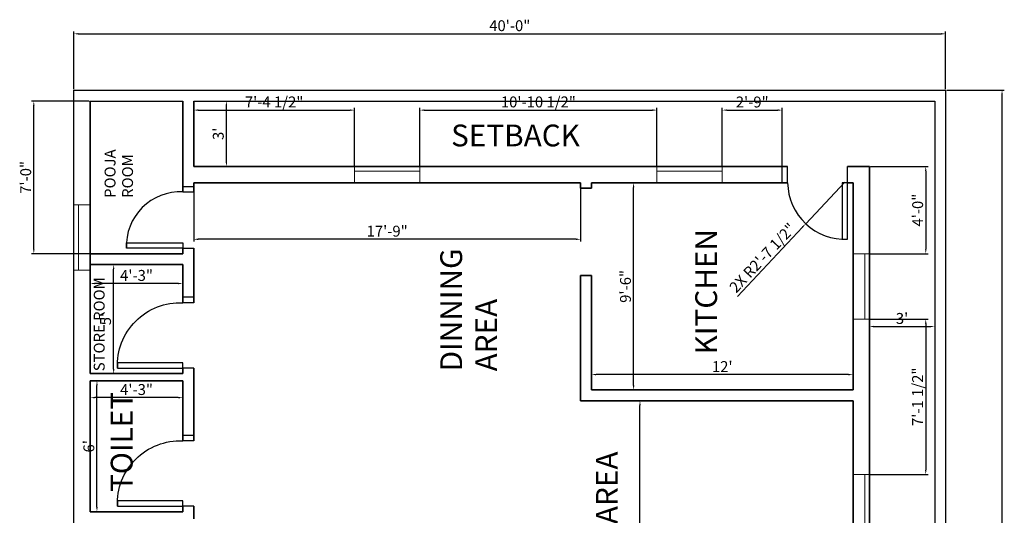
# Model space of a CAD drawing. Units: inches. Extents: x 2641 to 3210, y 2696 to 4064.
# Tile 2 of 4: x 2650 to 3192, y 3095 to 3367. Entities that reach past the tile are written whole.
import ezdxf

# ---------------------------------------------------------------- set-up
doc = ezdxf.new("R2010")
doc.units = ezdxf.units.IN
for name, color, linetype, lineweight in [('A-ANNO-DIMS', 2, 'Continuous', 18), ('A-AREA-IDEN', 7, 'Continuous', 18), ('A-DOOR', 3, 'Continuous', 25), ('A-GLAZ', 4, 'Continuous', 18), ('A-WALL', 7, 'Continuous', 35), ('C-PROP', 8, 'Continuous', 25)]:
    doc.layers.add(name, color=color, linetype=linetype, lineweight=lineweight)
doc.styles.get("Standard").update_dxf_attribs({"font": 'arial.ttf'})
doc.dimstyles.new('ISO-25', dxfattribs={"dimtxt": 6, "dimasz": 2.5, "dimexe": 1.25, "dimexo": 0.625, "dimtad": 1, "dimdec": 1, "dimlunit": 3, "dimtxsty": 'Standard', "dimcen": 2.5, "dimadec": 0, "dimazin": 0, "dimtfac": 1, "dimtdec": 1, "dimtmove": 0, "dimatfit": 3, "dimfxl": 1, "dimarcsym": 0})

# ---------------------------------------------------------------- blocks, each defined once
blk = doc.blocks.new('*D8')
at = {"layer": 'A-ANNO-DIMS', "color": 0, "lineweight": -2, "transparency": 16777216}
for p, q in [((2689.25, 3168.55), (2693.59, 3168.55)), ((2692.34, 3099.05), (2692.34, 3166.05)), ((2689.25, 3096.55), (2693.59, 3096.55))]:
    blk.add_line(p, q, dxfattribs=at)
at = {"layer": 'A-ANNO-DIMS', "color": 0, "transparency": 16777216}
for points in [[(2691.93, 3166.05), (2692.76, 3166.05), (2692.34, 3168.55)], [(2691.93, 3099.05), (2692.76, 3099.05), (2692.34, 3096.55)]]:
    blk.add_solid(points, dxfattribs=at)
at = {"layer": 'Defpoints', "color": 0, "transparency": 16777216}
for p in [(2688.63, 3168.55), (2692.34, 3168.55), (2688.63, 3096.55)]:
    blk.add_point(p, dxfattribs=at)
at = {"layer": 'A-ANNO-DIMS', "color": 0, "transparency": 16777216, "insert": (2688.65, 3132.55), "char_height": 6, "attachment_point": 5, "rotation": 90}
blk.add_mtext("6'", dxfattribs=at)
blk = doc.blocks.new('*D9')
at = {"layer": 'A-ANNO-DIMS', "color": 0, "lineweight": -2, "transparency": 16777216}
for p, q in [((2688.63, 3167.92), (2688.63, 3158.06)), ((2739.63, 3167.92), (2739.63, 3158.06)), ((2737.13, 3159.31), (2691.13, 3159.31))]:
    blk.add_line(p, q, dxfattribs=at)
at = {"layer": 'A-ANNO-DIMS', "color": 0, "transparency": 16777216}
for points in [[(2691.13, 3159.73), (2691.13, 3158.89), (2688.63, 3159.31)], [(2737.13, 3159.73), (2737.13, 3158.89), (2739.63, 3159.31)]]:
    blk.add_solid(points, dxfattribs=at)
at = {"layer": 'Defpoints', "color": 0, "transparency": 16777216}
for p in [(2688.63, 3168.55), (2739.63, 3168.55), (2688.63, 3159.31)]:
    blk.add_point(p, dxfattribs=at)
at = {"layer": 'A-ANNO-DIMS', "color": 0, "transparency": 16777216, "insert": (2714.13, 3163), "char_height": 6, "attachment_point": 5}
blk.add_mtext('4\'-3"', dxfattribs=at)
blk = doc.blocks.new('*D10')
at = {"layer": 'A-ANNO-DIMS', "color": 0, "lineweight": -2, "transparency": 16777216}
for p, q in [((2689.25, 3232.55), (2702.79, 3232.55)), ((2701.54, 3175.05), (2701.54, 3230.05)), ((2689.25, 3172.55), (2702.79, 3172.55))]:
    blk.add_line(p, q, dxfattribs=at)
at = {"layer": 'A-ANNO-DIMS', "color": 0, "transparency": 16777216}
for points in [[(2701.12, 3230.05), (2701.96, 3230.05), (2701.54, 3232.55)], [(2701.12, 3175.05), (2701.96, 3175.05), (2701.54, 3172.55)]]:
    blk.add_solid(points, dxfattribs=at)
at = {"layer": 'Defpoints', "color": 0, "transparency": 16777216}
for p in [(2688.63, 3232.55), (2701.54, 3232.55), (2688.63, 3172.55)]:
    blk.add_point(p, dxfattribs=at)
at = {"layer": 'A-ANNO-DIMS', "color": 0, "transparency": 16777216, "insert": (2697.86, 3202.55), "char_height": 6, "attachment_point": 5, "rotation": 90}
blk.add_mtext("5'", dxfattribs=at)
blk = doc.blocks.new('*D11')
at = {"layer": 'A-ANNO-DIMS', "color": 0, "lineweight": -2, "transparency": 16777216}
for p, q in [((2688.63, 3231.92), (2688.63, 3220.89)), ((2739.63, 3231.92), (2739.63, 3220.89)), ((2737.13, 3222.14), (2691.13, 3222.14))]:
    blk.add_line(p, q, dxfattribs=at)
at = {"layer": 'A-ANNO-DIMS', "color": 0, "transparency": 16777216}
for points in [[(2691.13, 3222.56), (2691.13, 3221.72), (2688.63, 3222.14)], [(2737.13, 3222.56), (2737.13, 3221.72), (2739.63, 3222.14)]]:
    blk.add_solid(points, dxfattribs=at)
at = {"layer": 'Defpoints', "color": 0, "transparency": 16777216}
for p in [(2688.63, 3232.55), (2739.63, 3232.55), (2688.63, 3222.14)]:
    blk.add_point(p, dxfattribs=at)
at = {"layer": 'A-ANNO-DIMS', "color": 0, "transparency": 16777216, "insert": (2714.13, 3225.83), "char_height": 6, "attachment_point": 5}
blk.add_mtext('4\'-3"', dxfattribs=at)
blk = doc.blocks.new('*D12')
at = {"layer": 'A-ANNO-DIMS', "color": 0, "lineweight": -2, "transparency": 16777216}
for p, q in [((2965.25, 3277.55), (2989.06, 3277.55)), ((2987.81, 3166.05), (2987.81, 3275.05)), ((2965.25, 3163.55), (2989.06, 3163.55))]:
    blk.add_line(p, q, dxfattribs=at)
at = {"layer": 'A-ANNO-DIMS', "color": 0, "transparency": 16777216}
for points in [[(2987.4, 3275.05), (2988.23, 3275.05), (2987.81, 3277.55)], [(2987.4, 3166.05), (2988.23, 3166.05), (2987.81, 3163.55)]]:
    blk.add_solid(points, dxfattribs=at)
at = {"layer": 'Defpoints', "color": 0, "transparency": 16777216}
for p in [(2964.63, 3277.55), (2987.81, 3277.55), (2964.63, 3163.55)]:
    blk.add_point(p, dxfattribs=at)
at = {"layer": 'A-ANNO-DIMS', "color": 0, "transparency": 16777216, "insert": (2984.12, 3220.55), "char_height": 6, "attachment_point": 5, "rotation": 90}
blk.add_mtext('9\'-6"', dxfattribs=at)
blk = doc.blocks.new('*D13')
at = {"layer": 'A-ANNO-DIMS', "color": 0, "lineweight": -2, "transparency": 16777216}
for p, q in [((2964.63, 3164.17), (2964.63, 3173.25)), ((3106.13, 3172), (2967.13, 3172)), ((3108.63, 3164.17), (3108.63, 3173.25))]:
    blk.add_line(p, q, dxfattribs=at)
at = {"layer": 'A-ANNO-DIMS', "color": 0, "transparency": 16777216}
for points in [[(2967.13, 3172.42), (2967.13, 3171.59), (2964.63, 3172)], [(3106.13, 3172.42), (3106.13, 3171.59), (3108.63, 3172)]]:
    blk.add_solid(points, dxfattribs=at)
at = {"layer": 'Defpoints', "color": 0, "transparency": 16777216}
for p in [(2964.63, 3172), (2964.63, 3163.55), (3108.63, 3163.55)]:
    blk.add_point(p, dxfattribs=at)
at = {"layer": 'A-ANNO-DIMS', "color": 0, "transparency": 16777216, "insert": (3036.63, 3175.64), "char_height": 6, "attachment_point": 5}
blk.add_mtext("12'", dxfattribs=at)
blk = doc.blocks.new('*D14')
at = {"layer": 'A-ANNO-DIMS', "color": 0, "lineweight": -2, "transparency": 16777216}
for p, q in [((2991, 3157.55), (2990.07, 3157.55)), ((2991.32, 2980.05), (2991.32, 3155.05)), ((2991, 2977.55), (2990.07, 2977.55))]:
    blk.add_line(p, q, dxfattribs=at)
at = {"layer": 'A-ANNO-DIMS', "color": 0, "transparency": 16777216}
for points in [[(2990.9, 3155.05), (2991.74, 3155.05), (2991.32, 3157.55)], [(2990.9, 2980.05), (2991.74, 2980.05), (2991.32, 2977.55)]]:
    blk.add_solid(points, dxfattribs=at)
at = {"layer": 'Defpoints', "color": 0, "transparency": 16777216}
for p in [(2991.32, 3157.55), (2991.63, 3157.55), (2991.63, 2977.55)]:
    blk.add_point(p, dxfattribs=at)
at = {"layer": 'A-ANNO-DIMS', "color": 0, "transparency": 16777216, "insert": (2987.63, 3067.55), "char_height": 6, "attachment_point": 5, "rotation": 90}
blk.add_mtext("15'", dxfattribs=at)
blk = doc.blocks.new('*D19')
at = {"layer": 'A-ANNO-DIMS', "color": 0, "lineweight": -2, "transparency": 16777216}
for p, q in [((2746.25, 3322.55), (2764.86, 3322.55)), ((2763.61, 3289.05), (2763.61, 3320.05)), ((2746.25, 3286.55), (2764.86, 3286.55))]:
    blk.add_line(p, q, dxfattribs=at)
at = {"layer": 'A-ANNO-DIMS', "color": 0, "transparency": 16777216}
for points in [[(2763.19, 3320.05), (2764.02, 3320.05), (2763.61, 3322.55)], [(2763.19, 3289.05), (2764.02, 3289.05), (2763.61, 3286.55)]]:
    blk.add_solid(points, dxfattribs=at)
at = {"layer": 'Defpoints', "color": 0, "transparency": 16777216}
for p in [(2745.63, 3322.55), (2763.61, 3322.55), (2745.63, 3286.55)]:
    blk.add_point(p, dxfattribs=at)
at = {"layer": 'A-ANNO-DIMS', "color": 0, "transparency": 16777216, "insert": (2759.92, 3304.55), "char_height": 6, "attachment_point": 5, "rotation": 90}
blk.add_mtext("3'", dxfattribs=at)
blk = doc.blocks.new('*D20')
at = {"layer": 'A-ANNO-DIMS', "color": 0, "lineweight": -2, "transparency": 16777216}
for p, q in [((3117.63, 3285.92), (3117.63, 3197.2)), ((3153.63, 3285.92), (3153.63, 3197.2)), ((3120.13, 3198.45), (3151.13, 3198.45))]:
    blk.add_line(p, q, dxfattribs=at)
at = {"layer": 'A-ANNO-DIMS', "color": 0, "transparency": 16777216}
for points in [[(3120.13, 3198.87), (3120.13, 3198.03), (3117.63, 3198.45)], [(3151.13, 3198.87), (3151.13, 3198.03), (3153.63, 3198.45)]]:
    blk.add_solid(points, dxfattribs=at)
at = {"layer": 'Defpoints', "color": 0, "transparency": 16777216}
for p in [(3117.63, 3286.55), (3153.63, 3286.55), (3153.63, 3198.45)]:
    blk.add_point(p, dxfattribs=at)
at = {"layer": 'A-ANNO-DIMS', "color": 0, "transparency": 16777216, "insert": (3135.63, 3202.14), "char_height": 6, "attachment_point": 5}
blk.add_mtext("3'", dxfattribs=at)
blk = doc.blocks.new('DOOR-36-INT')
for p, q in [((0, 42.03), (0, 36.03)), ((36, 42.03), (36, 36.03)), ((39, 42.03), (39, 36.03))]:
    blk.add_line(p, q)
blk.add_lwpolyline([(0, 36.03), (3, 36.03), (3, 0.03), (0, 0.03)], close=True)
blk.add_arc((1.5, 34.53), 34.53, 267.5104, 2.4896)
blk = doc.blocks.new('DOOR-31-INT')
for p, q in [((31.04, 34), (37.04, 34)), ((31.04, 31), (37.04, 31)), ((31.04, 0), (37.04, 0))]:
    blk.add_line(p, q)
blk.add_lwpolyline([(31.04, 0), (0.04, 0), (0.04, 3), (31.04, 3)], close=True)
blk.add_arc((29.54, 1.5), 29.54, 87.0892, 182.9108)
blk = doc.blocks.new('DOOR-31-EXT')
for p, q in [((0, 31.04), (0, 40.04)), ((3, 31.04), (3, 40.04))]:
    blk.add_line(p, q)
blk.add_lwpolyline([(36, 31.04), (33, 31.04), (33, 0.04), (36, 0.04)], close=True)
blk.add_arc((34.5, 31.5), 31.5, 180.8507, 272.7291)
blk = doc.blocks.new('WIN-36x9')
blk.add_line((6.5, 36), (6.5, 0))
blk.add_lwpolyline([(9, 36), (0, 36), (0, 0), (9, 0)], close=True)
blk = doc.blocks.new('*D51')
at = {"layer": 'A-ANNO-DIMS', "color": 0, "lineweight": -2, "transparency": 16777216}
for p, q in [((2679.63, 3329.17), (2679.63, 3360.85)), ((2682.13, 3359.6), (3157.13, 3359.6)), ((3159.63, 3329.17), (3159.63, 3360.85))]:
    blk.add_line(p, q, dxfattribs=at)
at = {"layer": 'A-ANNO-DIMS', "color": 0, "transparency": 16777216}
for points in [[(2682.13, 3360.02), (2682.13, 3359.18), (2679.63, 3359.6)], [(3157.13, 3360.02), (3157.13, 3359.18), (3159.63, 3359.6)]]:
    blk.add_solid(points, dxfattribs=at)
at = {"layer": 'Defpoints', "color": 0, "transparency": 16777216}
for p in [(3159.63, 3359.6), (2679.63, 3328.55), (3159.63, 3328.55)]:
    blk.add_point(p, dxfattribs=at)
at = {"layer": 'A-ANNO-DIMS', "color": 0, "transparency": 16777216, "insert": (2919.63, 3363.29), "char_height": 6, "attachment_point": 5}
blk.add_mtext('40\'-0"', dxfattribs=at)
blk = doc.blocks.new('*D52')
at = {"layer": 'A-ANNO-DIMS', "color": 0, "lineweight": -2, "transparency": 16777216}
for p, q in [((3160.25, 3328.55), (3191.93, 3328.55)), ((3190.68, 2731.05), (3190.68, 3326.05)), ((3160.25, 2728.55), (3191.93, 2728.55))]:
    blk.add_line(p, q, dxfattribs=at)
at = {"layer": 'A-ANNO-DIMS', "color": 0, "transparency": 16777216}
for points in [[(3190.26, 3326.05), (3191.09, 3326.05), (3190.68, 3328.55)], [(3190.26, 2731.05), (3191.09, 2731.05), (3190.68, 2728.55)]]:
    blk.add_solid(points, dxfattribs=at)
at = {"layer": 'Defpoints', "color": 0, "transparency": 16777216}
for p in [(3159.63, 3328.55), (3190.68, 3328.55), (3159.63, 2728.55)]:
    blk.add_point(p, dxfattribs=at)
at = {"layer": 'A-ANNO-DIMS', "color": 0, "transparency": 16777216, "insert": (3186.99, 3028.55), "char_height": 6, "attachment_point": 5, "rotation": 90}
blk.add_mtext('50\'-0"', dxfattribs=at)
blk = doc.blocks.new('*D57')
at = {"layer": 'A-ANNO-DIMS', "color": 0, "lineweight": -2, "transparency": 16777216}
for p, q in [((2745.63, 3276.92), (2745.63, 3245.25)), ((2958.63, 3276.92), (2958.63, 3245.25)), ((2956.13, 3246.5), (2748.13, 3246.5))]:
    blk.add_line(p, q, dxfattribs=at)
at = {"layer": 'A-ANNO-DIMS', "color": 0, "transparency": 16777216}
for points in [[(2748.13, 3246.92), (2748.13, 3246.08), (2745.63, 3246.5)], [(2956.13, 3246.92), (2956.13, 3246.08), (2958.63, 3246.5)]]:
    blk.add_solid(points, dxfattribs=at)
at = {"layer": 'Defpoints', "color": 0, "transparency": 16777216}
for p in [(2745.63, 3277.55), (2958.63, 3277.55), (2745.63, 3246.5)]:
    blk.add_point(p, dxfattribs=at)
at = {"layer": 'A-ANNO-DIMS', "color": 0, "transparency": 16777216, "insert": (2852.13, 3250.19), "char_height": 6, "attachment_point": 5}
blk.add_mtext('17\'-9"', dxfattribs=at)
blk = doc.blocks.new('*D58')
at = {"layer": 'A-ANNO-DIMS', "color": 0, "lineweight": -2, "transparency": 16777216}
for p, q in [((2688, 3322.55), (2656.33, 3322.55)), ((2657.58, 3241.05), (2657.58, 3320.05)), ((2688, 3238.55), (2656.33, 3238.55))]:
    blk.add_line(p, q, dxfattribs=at)
at = {"layer": 'A-ANNO-DIMS', "color": 0, "transparency": 16777216}
for points in [[(2657.16, 3320.05), (2657.99, 3320.05), (2657.58, 3322.55)], [(2657.16, 3241.05), (2657.99, 3241.05), (2657.58, 3238.55)]]:
    blk.add_solid(points, dxfattribs=at)
at = {"layer": 'Defpoints', "color": 0, "transparency": 16777216}
for p in [(2657.58, 3322.55), (2688.63, 3322.55), (2688.63, 3238.55)]:
    blk.add_point(p, dxfattribs=at)
at = {"layer": 'A-ANNO-DIMS', "color": 0, "transparency": 16777216, "insert": (2653.89, 3280.55), "char_height": 6, "attachment_point": 5, "rotation": 90}
blk.add_mtext('7\'-0"', dxfattribs=at)
blk = doc.blocks.new('*D59')
at = {"layer": 'A-ANNO-DIMS', "color": 0, "lineweight": -2, "transparency": 16777216}
for p, q in [((2745.63, 3287.17), (2745.63, 3318.85)), ((2834.13, 3287.17), (2834.13, 3318.85)), ((2748.13, 3317.6), (2831.63, 3317.6))]:
    blk.add_line(p, q, dxfattribs=at)
at = {"layer": 'A-ANNO-DIMS', "color": 0, "transparency": 16777216}
for points in [[(2748.13, 3318.02), (2748.13, 3317.18), (2745.63, 3317.6)], [(2831.63, 3318.02), (2831.63, 3317.18), (2834.13, 3317.6)]]:
    blk.add_solid(points, dxfattribs=at)
at = {"layer": 'Defpoints', "color": 0, "transparency": 16777216}
for p in [(2834.13, 3317.6), (2745.63, 3286.55), (2834.13, 3286.55)]:
    blk.add_point(p, dxfattribs=at)
at = {"layer": 'A-ANNO-DIMS', "color": 0, "transparency": 16777216, "insert": (2789.88, 3321.33), "char_height": 6, "attachment_point": 5}
blk.add_mtext('7\'-4 1/2"', dxfattribs=at)
blk = doc.blocks.new('*D60')
at = {"layer": 'A-ANNO-DIMS', "color": 0, "lineweight": -2, "transparency": 16777216}
for p, q in [((2870.13, 3287.17), (2870.13, 3318.85)), ((3000.63, 3287.17), (3000.63, 3318.85)), ((2872.63, 3317.6), (2998.13, 3317.6))]:
    blk.add_line(p, q, dxfattribs=at)
at = {"layer": 'A-ANNO-DIMS', "color": 0, "transparency": 16777216}
for points in [[(2872.63, 3318.02), (2872.63, 3317.18), (2870.13, 3317.6)], [(2998.13, 3318.02), (2998.13, 3317.18), (3000.63, 3317.6)]]:
    blk.add_solid(points, dxfattribs=at)
at = {"layer": 'Defpoints', "color": 0, "transparency": 16777216}
for p in [(3000.63, 3317.6), (2870.13, 3286.55), (3000.63, 3286.55)]:
    blk.add_point(p, dxfattribs=at)
at = {"layer": 'A-ANNO-DIMS', "color": 0, "transparency": 16777216, "insert": (2935.38, 3321.33), "char_height": 6, "attachment_point": 5}
blk.add_mtext('10\'-10 1/2"', dxfattribs=at)
blk = doc.blocks.new('*D61')
at = {"layer": 'A-ANNO-DIMS', "color": 0, "lineweight": -2, "transparency": 16777216}
for p, q in [((3036.63, 3287.17), (3036.63, 3318.85)), ((3069.63, 3287.17), (3069.63, 3318.85)), ((3039.13, 3317.6), (3067.13, 3317.6))]:
    blk.add_line(p, q, dxfattribs=at)
at = {"layer": 'A-ANNO-DIMS', "color": 0, "transparency": 16777216}
for points in [[(3039.13, 3318.02), (3039.13, 3317.18), (3036.63, 3317.6)], [(3067.13, 3318.02), (3067.13, 3317.18), (3069.63, 3317.6)]]:
    blk.add_solid(points, dxfattribs=at)
at = {"layer": 'Defpoints', "color": 0, "transparency": 16777216}
for p in [(3069.63, 3317.6), (3036.63, 3286.55), (3069.63, 3286.55)]:
    blk.add_point(p, dxfattribs=at)
at = {"layer": 'A-ANNO-DIMS', "color": 0, "transparency": 16777216, "insert": (3053.13, 3321.29), "char_height": 6, "attachment_point": 5}
blk.add_mtext('2\'-9"', dxfattribs=at)
blk = doc.blocks.new('*D62')
at = {"layer": 'A-ANNO-DIMS', "color": 0, "lineweight": -2, "transparency": 16777216}
for p, q in [((3118.25, 3202.55), (3149.93, 3202.55)), ((3148.68, 3200.05), (3148.68, 3119.55)), ((3118.25, 3117.05), (3149.93, 3117.05))]:
    blk.add_line(p, q, dxfattribs=at)
at = {"layer": 'A-ANNO-DIMS', "color": 0, "transparency": 16777216}
for points in [[(3148.26, 3200.05), (3149.09, 3200.05), (3148.68, 3202.55)], [(3148.26, 3119.55), (3149.09, 3119.55), (3148.68, 3117.05)]]:
    blk.add_solid(points, dxfattribs=at)
at = {"layer": 'Defpoints', "color": 0, "transparency": 16777216}
for p in [(3117.63, 3202.55), (3117.63, 3117.05), (3148.68, 3117.05)]:
    blk.add_point(p, dxfattribs=at)
at = {"layer": 'A-ANNO-DIMS', "color": 0, "transparency": 16777216, "insert": (3144.95, 3159.8), "char_height": 6, "attachment_point": 5, "rotation": 90}
blk.add_mtext('7\'-1 1/2"', dxfattribs=at)
blk = doc.blocks.new('*D63')
at = {"layer": 'A-ANNO-DIMS', "color": 0, "lineweight": -2, "transparency": 16777216}
for p, q in [((3118.25, 3286.55), (3149.93, 3286.55)), ((3148.68, 3284.05), (3148.68, 3241.05)), ((3118.25, 3238.55), (3149.93, 3238.55))]:
    blk.add_line(p, q, dxfattribs=at)
at = {"layer": 'A-ANNO-DIMS', "color": 0, "transparency": 16777216}
for points in [[(3148.26, 3284.05), (3149.09, 3284.05), (3148.68, 3286.55)], [(3148.26, 3241.05), (3149.09, 3241.05), (3148.68, 3238.55)]]:
    blk.add_solid(points, dxfattribs=at)
at = {"layer": 'Defpoints', "color": 0, "transparency": 16777216}
for p in [(3117.63, 3286.55), (3117.63, 3238.55), (3148.68, 3238.55)]:
    blk.add_point(p, dxfattribs=at)
at = {"layer": 'A-ANNO-DIMS', "color": 0, "transparency": 16777216, "insert": (3144.99, 3262.55), "char_height": 6, "attachment_point": 5, "rotation": 90}
blk.add_mtext('4\'-0"', dxfattribs=at)
blk = doc.blocks.new('*D87')
at = {"layer": 'A-ANNO-DIMS', "color": 0, "lineweight": -2, "transparency": 16777216}
for p, q in [((3104.13, 3278.02), (3082.56, 3255.06)), ((3044.96, 3215.03), (3080.84, 3253.23))]:
    blk.add_line(p, q, dxfattribs=at)
at = {"layer": 'A-ANNO-DIMS', "color": 0, "transparency": 16777216}
blk.add_solid([(3080.54, 3253.52), (3081.15, 3252.95), (3082.56, 3255.06)], dxfattribs=at)
at = {"layer": 'Defpoints', "color": 0, "transparency": 16777216}
for p in [(3104.13, 3278.02), (3082.56, 3255.06)]:
    blk.add_point(p, dxfattribs=at)
at = {"layer": 'A-ANNO-DIMS', "color": 0, "transparency": 16777216, "insert": (3059.33, 3235.77), "char_height": 6, "attachment_point": 5, "rotation": 46.7899}
blk.add_mtext('2X R2\'-7 1/2"', dxfattribs=at)

msp = doc.modelspace()

# ---------------------------------------------------------------- linework, layer by layer
at = {"layer": 'A-DOOR'}
msp.add_line((3105.63, 3277.55), (3105.63, 3286.55), dxfattribs=at)
at = {"layer": 'A-WALL'}
for p, q in [((2688.63, 3172.55), (2688.63, 3322.55)), ((2739.63, 3272.55), (2739.63, 3322.55)), ((2745.63, 3286.55), (2745.63, 3322.55)), ((2745.63, 3277.55), (2958.63, 3277.55)), ((2745.63, 3272.55), (2745.63, 3277.55)), ((2958.63, 3277.55), (2958.63, 3274.55)), ((2958.63, 3277.55), (2958.63, 3274.55)), ((2958.63, 3274.55), (2964.63, 3274.55)), ((2964.63, 3277.55), (2964.63, 3274.55)), ((2964.63, 3277.55), (3072.63, 3277.55)), ((3108.63, 3277.55), (3105.63, 3277.55)), ((3105.63, 3277.55), (3108.63, 3277.55)), ((3108.63, 3277.55), (3108.63, 3163.55)), ((2688.63, 3238.55), (2739.63, 3238.55)), ((2739.63, 3238.55), (2739.63, 3241.55)), ((2739.63, 3238.55), (2739.63, 3241.55)), ((2745.63, 3211.55), (2745.63, 3241.55)), ((2688.63, 3232.55), (2739.63, 3232.55)), ((2739.63, 3211.55), (2739.63, 3232.55)), ((2958.63, 3226.55), (2964.63, 3226.55)), ((2958.63, 3226.55), (2958.63, 3157.55)), ((2964.63, 3226.55), (2964.63, 3163.55)), ((2688.63, 3172.55), (2739.63, 3172.55)), ((2739.63, 3172.55), (2739.63, 3175.55)), ((2739.63, 3172.55), (2739.63, 3175.55)), ((2745.63, 3135.55), (2745.63, 3175.55)), ((2688.63, 3168.55), (2739.63, 3168.55)), ((2688.63, 3096.55), (2688.63, 3168.55)), ((2739.63, 3135.55), (2739.63, 3168.55)), ((3108.63, 3163.55), (2964.63, 3163.55)), ((2688.63, 3096.55), (2688.63, 3157.55)), ((3108.63, 3157.55), (2958.63, 3157.55)), ((3108.63, 3157.55), (3108.63, 3040.55)), ((2688.63, 3096.55), (2739.63, 3096.55)), ((2739.63, 3096.55), (2739.63, 3099.55)), ((2739.63, 3096.55), (2739.63, 3099.55)), ((2745.63, 3092.55), (2745.63, 3099.55))]:
    msp.add_line(p, q, dxfattribs=at)
for points in [[(2745.63, 3286.55), (3072.63, 3286.55)], [(3105.63, 3286.55), (3117.63, 3286.55), (3117.63, 3040.55)]]:
    msp.add_lwpolyline(points, dxfattribs=at)
at = {"layer": 'C-PROP'}
for p, q in [((2679.63, 2728.55), (2679.63, 3328.55)), ((2679.63, 3328.55), (3159.63, 3328.55)), ((3159.63, 3328.55), (3159.63, 2728.55)), ((2688.63, 3322.55), (2739.63, 3322.55)), ((2745.63, 3322.55), (3153.63, 3322.55)), ((3153.63, 3322.55), (3153.63, 2968.55))]:
    msp.add_line(p, q, dxfattribs=at)

# ---------------------------------------------------------------- block references
at = {"layer": 'A-DOOR'}
for name, p in [('DOOR-31-EXT', (3069.63, 3246.51)), ('DOOR-31-INT', (2708.59, 3241.55))]:
    msp.add_blockref(name, p, dxfattribs=at)
at = {"layer": 'A-DOOR', "extrusion": (0, 0, -1), "zscale": -1, "rotation": 89.99999999999825}
for p in [(-2703.59, 3175.55), (-2703.59, 3099.55)]:
    msp.add_blockref('DOOR-36-INT', p, dxfattribs=at)
at = {"layer": 'A-GLAZ'}
for p, rotation in [((2870.13, 3277.55), 90.0000000000012), ((3036.63, 3277.55), 90.00000000000183), ((2688.63, 3265.55), 180)]:
    msp.add_blockref('WIN-36x9', p, dxfattribs=dict(at, rotation=rotation))
for p in [(3108.63, 3202.55), (3108.63, 3081.05)]:
    msp.add_blockref('WIN-36x9', p, dxfattribs=at)

# ---------------------------------------------------------------- texts
at = {"layer": 'A-AREA-IDEN'}
msp.add_text('SETBACK', height=12, dxfattribs=at).set_placement((2887.33, 3297.64))
for s, height, p in [('POOJA', 6, (2702.56, 3269.3)), ('ROOM', 6, (2712.19, 3269.3)), ('KITCHEN', 12, (3033.77, 3183.11)), ('DINNING', 12, (2893.39, 3173.78)), ('STORE ROOM', 6, (2696.57, 3173.86)), ('AREA', 12, (2912.67, 3173.78)), ('TOILET', 12, (2711.95, 3107.38)), ('HALL/LIVING AREA', 12, (2979.08, 2988.98))]:
    msp.add_text(s, height=height, rotation=90, dxfattribs=at).set_placement(p)

# ---------------------------------------------------------------- dimensions: what is measured, and where the dimension line sits
at = {"layer": 'A-ANNO-DIMS'}
for base, p1, p2, override, picture, middle in [((3159.63, 3359.6), (2679.63, 3328.55), (3159.63, 3328.55), {"dimdec": 1, "dimlfac": 1, "dimrnd": 0, "dimzin": 1, "dimdsep": 46, "dimlunit": 4, "dimfrac": 2}, '*D51', (2919.63, 3363.29)), ((2834.13, 3317.6), (2745.63, 3286.55), (2834.13, 3286.55), {"dimdec": 1, "dimlfac": 1, "dimrnd": 0, "dimzin": 1, "dimdsep": 46, "dimlunit": 4, "dimfrac": 2}, '*D59', (2789.88, 3321.33)), ((3000.63, 3317.6), (2870.13, 3286.55), (3000.63, 3286.55), {"dimdec": 1, "dimlfac": 1, "dimrnd": 0, "dimzin": 1, "dimdsep": 46, "dimlunit": 4, "dimfrac": 2}, '*D60', (2935.38, 3321.33)), ((3069.63, 3317.6), (3036.63, 3286.55), (3069.63, 3286.55), {"dimdec": 1, "dimlfac": 1, "dimrnd": 0, "dimzin": 1, "dimdsep": 46, "dimlunit": 4, "dimfrac": 2}, '*D61', (3053.13, 3321.29)), ((3153.63, 3198.45), (3117.63, 3286.55), (3153.63, 3286.55), {"dimclrd": 0, "dimclre": 0, "dimclrt": 0}, '*D20', (3135.63, 3202.14)), ((2688.63, 3222.14), (2739.63, 3232.55), (2688.63, 3232.55), {"dimclrd": 0, "dimclre": 0, "dimclrt": 0}, '*D11', (2714.13, 3225.83)), ((2964.63, 3172), (3108.63, 3163.55), (2964.63, 3163.55), {"dimclrd": 0, "dimclre": 0, "dimclrt": 0}, '*D13', (3036.63, 3175.64)), ((2688.63, 3159.31), (2739.63, 3168.55), (2688.63, 3168.55), {"dimclrd": 0, "dimclre": 0, "dimclrt": 0}, '*D9', (2714.13, 3163))]:
    dim = msp.add_linear_dim(base=base, p1=p1, p2=p2, dimstyle='ISO-25', override=override, dxfattribs=at)
    dim.commit()
    dim.dimension.update_dxf_attribs({"geometry": picture, "text_midpoint": middle})
for base, p1, p2, angle, override, picture, middle in [((3190.68, 3328.55), (3159.63, 2728.55), (3159.63, 3328.55), 90, {"dimdec": 1, "dimlfac": 1, "dimrnd": 0, "dimzin": 1, "dimdsep": 46, "dimlunit": 4, "dimfrac": 2}, '*D52', (3186.99, 3028.55)), ((2657.58, 3322.55), (2688.63, 3238.55), (2688.63, 3322.55), 90, {"dimdec": 1, "dimlfac": 1, "dimrnd": 0, "dimzin": 1, "dimdsep": 46, "dimlunit": 4, "dimfrac": 2}, '*D58', (2653.89, 3280.55)), ((2763.61, 3322.55), (2745.63, 3286.55), (2745.63, 3322.55), 90, {"dimclrd": 0, "dimclre": 0, "dimclrt": 0}, '*D19', (2759.92, 3304.55)), ((3148.68, 3238.55), (3117.63, 3286.55), (3117.63, 3238.55), 270, {"dimdec": 1, "dimlfac": 1, "dimrnd": 0, "dimzin": 1, "dimdsep": 46, "dimlunit": 4, "dimfrac": 2}, '*D63', (3144.99, 3262.55)), ((2745.63, 3246.5), (2958.63, 3277.55), (2745.63, 3277.55), 180, {"dimdec": 1, "dimlfac": 1, "dimrnd": 0, "dimzin": 1, "dimdsep": 46, "dimlunit": 4, "dimfrac": 2}, '*D57', (2852.13, 3250.19)), ((2987.81, 3277.55), (2964.63, 3163.55), (2964.63, 3277.55), 90, {"dimclrd": 0, "dimclre": 0, "dimclrt": 0}, '*D12', (2984.12, 3220.55)), ((2701.54, 3232.55), (2688.63, 3172.55), (2688.63, 3232.55), 90, {"dimclrd": 0, "dimclre": 0, "dimclrt": 0}, '*D10', (2697.86, 3202.55)), ((3148.68, 3117.05), (3117.63, 3202.55), (3117.63, 3117.05), 270, {"dimdec": 1, "dimlfac": 1, "dimrnd": 0, "dimzin": 1, "dimdsep": 46, "dimlunit": 4, "dimfrac": 2}, '*D62', (3144.95, 3159.8)), ((2692.34, 3168.55), (2688.63, 3096.55), (2688.63, 3168.55), 90, {"dimclrd": 0, "dimclre": 0, "dimclrt": 0}, '*D8', (2688.65, 3132.55)), ((2991.32, 3157.55), (2991.63, 2977.55), (2991.63, 3157.55), 90, {"dimclrd": 0, "dimclre": 0, "dimclrt": 0}, '*D14', (2987.63, 3067.55))]:
    dim = msp.add_linear_dim(base=base, p1=p1, p2=p2, angle=angle, dimstyle='ISO-25', override=override, dxfattribs=at)
    dim.commit()
    dim.dimension.update_dxf_attribs({"geometry": picture, "text_midpoint": middle})
dim = msp.add_radius_dim(center=(3104.13, 3278.02), mpoint=(3082.56, 3255.06), text='2X <>', dimstyle='ISO-25', override={"dimdec": 1, "dimlfac": 1, "dimrnd": 0, "dimzin": 1, "dimdsep": 46, "dimlunit": 4, "dimfrac": 2}, dxfattribs=at)
dim.commit()
dim.dimension.update_dxf_attribs({"geometry": '*D87', "text_midpoint": (3059.33, 3235.77)})

doc.saveas('drawing.dxf')
